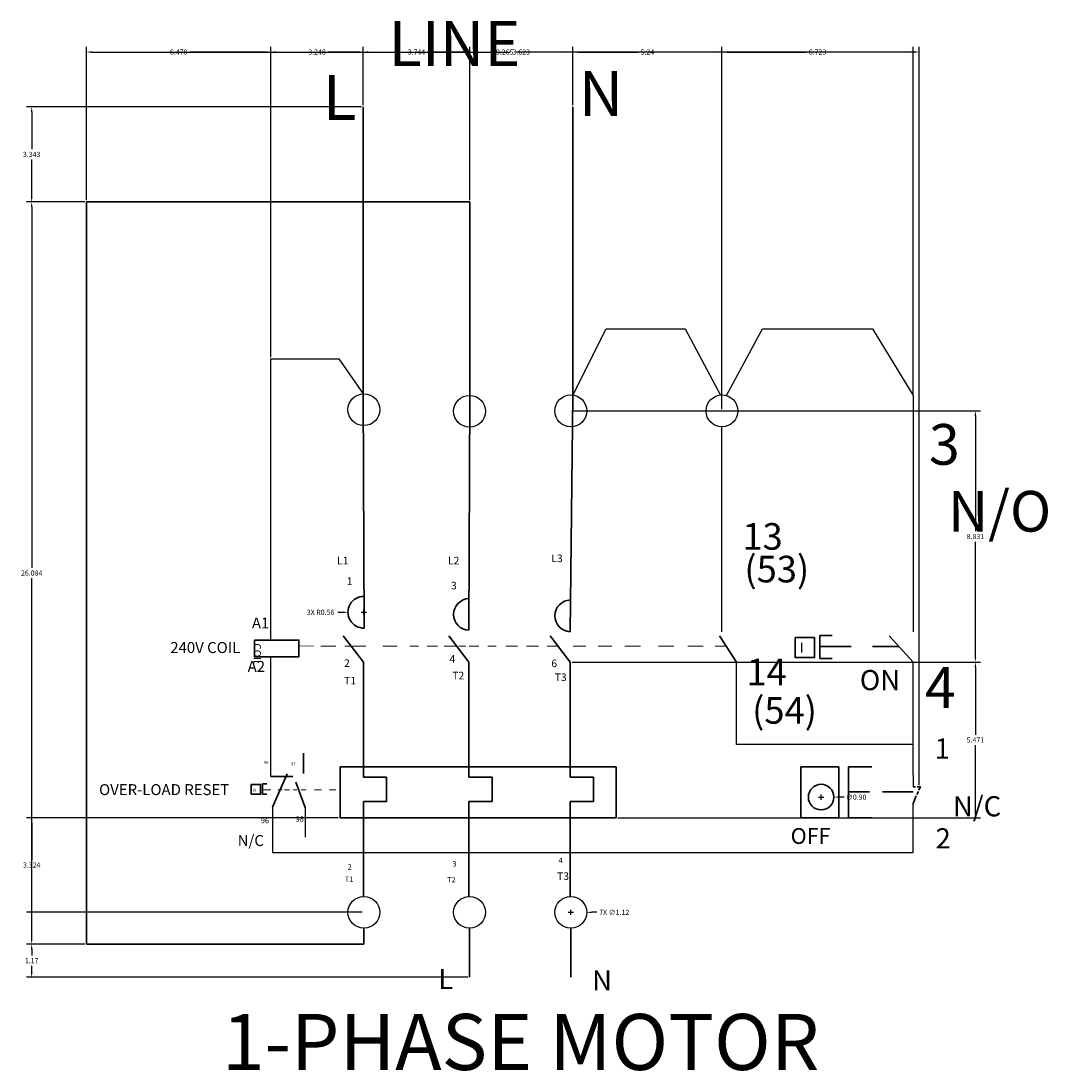
# Model space of a CAD drawing. Units: inches. Extents: x 14.6 to 50.7, y 1.8 to 38.7.
import ezdxf

# ---------------------------------------------------------------- set-up
doc = ezdxf.new("R2010")
doc.units = ezdxf.units.IN
doc.header["$MEASUREMENT"] = 0
for name, color, linetype, lineweight in [('A-ANNO-DIMS', 2, 'Continuous', 18), ('E-ANNO-TEXT', 7, 'Continuous', 18), ('E-CTRL-PBTN', 7, 'Continuous', 30), ('E-CTRL-WIRE', 4, 'Continuous', 25), ('E-EQPM-LINK', 8, 'Continuous', 18), ('E-POWR-CONT', 7, 'Continuous', 30), ('E-POWR-OVLD', 7, 'Continuous', 30), ('E-POWR-TERM', 2, 'Continuous', 25), ('E-POWR-WIRE', 1, 'Continuous', 35)]:
    doc.layers.add(name, color=color, linetype=linetype, lineweight=lineweight)
doc.styles.get("Standard").update_dxf_attribs({"font": 'arial.ttf'})
doc.dimstyles.get("Standard").update_dxf_attribs({"dimtxt": 0.18, "dimasz": 0.18, "dimexe": 0.18, "dimexo": 0.0625, "dimgap": 0.09, "dimtad": 0, "dimtih": 1, "dimtoh": 1, "dimdec": 4, "dimzin": 0, "dimdsep": 46, "dimtxsty": 'Standard', "dimcen": 0.09, "dimadec": 0, "dimazin": 0, "dimtfac": 1, "dimtdec": 4, "dimtofl": 0, "dimtmove": 0, "dimatfit": 3, "dimfxl": 1, "dimtolj": 1, "dimtzin": 0, "dimarcsym": 0})

# ---------------------------------------------------------------- blocks, each defined once
blk = doc.blocks.new('OL-HEATER-ELEMENT')
for p, q in [((0.817, 0.861), (0, 0.861)), ((0.817, 0), (0.817, 0.861)), ((0, 0), (0.817, 0))]:
    blk.add_line(p, q)
blk = doc.blocks.new('WIRING-TERMINAL')
blk.add_circle((0, 0), 0.558)
blk = doc.blocks.new('*D3')
at = {"layer": 'A-ANNO-DIMS', "color": 0, "lineweight": -2, "transparency": 16777216}
for p, q in [((16.913, 32.366), (16.913, 37.754)), ((46.178, 11.804), (46.178, 37.754)), ((17.093, 37.574), (31.08, 37.574)), ((45.998, 37.574), (32.011, 37.574))]:
    blk.add_line(p, q, dxfattribs=at)
at = {"layer": 'A-ANNO-DIMS', "color": 0, "transparency": 16777216}
for points in [[(17.093, 37.604), (17.093, 37.544), (16.913, 37.574)], [(45.998, 37.604), (45.998, 37.544), (46.178, 37.574)]]:
    blk.add_solid(points, dxfattribs=at)
at = {"layer": 'Defpoints', "color": 0, "transparency": 16777216}
for p in [(46.178, 37.574), (16.913, 32.303), (46.178, 11.741)]:
    blk.add_point(p, dxfattribs=at)
at = {"layer": 'A-ANNO-DIMS', "color": 0, "transparency": 16777216, "insert": (31.546, 37.574), "char_height": 0.18, "attachment_point": 5}
blk.add_mtext('\\A1;29.265', dxfattribs=at)
blk = doc.blocks.new('*D4')
at = {"layer": 'A-ANNO-DIMS', "color": 0, "lineweight": -2, "transparency": 16777216}
for p, q in [((16.851, 32.303), (14.806, 32.303)), ((14.986, 32.123), (14.986, 19.443)), ((14.986, 6.399), (14.986, 19.079)), ((16.851, 6.219), (14.806, 6.219))]:
    blk.add_line(p, q, dxfattribs=at)
at = {"layer": 'A-ANNO-DIMS', "color": 0, "transparency": 16777216}
for points in [[(14.956, 32.123), (15.016, 32.123), (14.986, 32.303)], [(14.956, 6.399), (15.016, 6.399), (14.986, 6.219)]]:
    blk.add_solid(points, dxfattribs=at)
at = {"layer": 'Defpoints', "color": 0, "transparency": 16777216}
for p in [(14.986, 32.303), (16.913, 32.303), (16.913, 6.219)]:
    blk.add_point(p, dxfattribs=at)
at = {"layer": 'A-ANNO-DIMS', "color": 0, "transparency": 16777216, "insert": (14.986, 19.261), "char_height": 0.18, "attachment_point": 5}
blk.add_mtext('\\A1;26.084', dxfattribs=at)
blk = doc.blocks.new('*D5')
at = {"layer": 'A-ANNO-DIMS', "color": 0, "lineweight": -2, "transparency": 16777216}
for p, q in [((26.576, 35.647), (14.806, 35.647)), ((14.986, 35.467), (14.986, 34.157)), ((14.986, 32.483), (14.986, 33.793)), ((16.851, 32.303), (14.806, 32.303))]:
    blk.add_line(p, q, dxfattribs=at)
at = {"layer": 'A-ANNO-DIMS', "color": 0, "transparency": 16777216}
for points in [[(14.956, 35.467), (15.016, 35.467), (14.986, 35.647)], [(14.956, 32.483), (15.016, 32.483), (14.986, 32.303)]]:
    blk.add_solid(points, dxfattribs=at)
at = {"layer": 'Defpoints', "color": 0, "transparency": 16777216}
for p in [(14.986, 35.647), (26.639, 35.647), (16.913, 32.303)]:
    blk.add_point(p, dxfattribs=at)
at = {"layer": 'A-ANNO-DIMS', "color": 0, "transparency": 16777216, "insert": (14.986, 33.975), "char_height": 0.18, "attachment_point": 5}
blk.add_mtext('\\A1;3.343', dxfattribs=at)
blk = doc.blocks.new('*D6')
at = {"layer": 'A-ANNO-DIMS', "color": 0, "lineweight": -2, "transparency": 16777216}
for p, q in [((16.851, 6.219), (14.806, 6.219)), ((14.986, 6.039), (14.986, 5.816)), ((14.986, 5.233), (14.986, 5.456)), ((30.313, 5.053), (14.806, 5.053))]:
    blk.add_line(p, q, dxfattribs=at)
at = {"layer": 'A-ANNO-DIMS', "color": 0, "transparency": 16777216}
for points in [[(14.956, 6.039), (15.016, 6.039), (14.986, 6.219)], [(14.956, 5.233), (15.016, 5.233), (14.986, 5.053)]]:
    blk.add_solid(points, dxfattribs=at)
at = {"layer": 'Defpoints', "color": 0, "transparency": 16777216}
for p in [(14.986, 6.219), (16.913, 6.219), (30.375, 5.053)]:
    blk.add_point(p, dxfattribs=at)
at = {"layer": 'A-ANNO-DIMS', "color": 0, "transparency": 16777216, "insert": (14.986, 5.636), "char_height": 0.18, "attachment_point": 5}
blk.add_mtext('\\A1;1.17', dxfattribs=at)
blk = doc.blocks.new('*D7')
at = {"layer": 'A-ANNO-DIMS', "color": 0, "lineweight": -2, "transparency": 16777216}
for p, q in [((16.913, 32.366), (16.913, 37.754)), ((23.391, 26.852), (23.391, 37.754)), ((17.093, 37.574), (19.758, 37.574)), ((23.211, 37.574), (20.546, 37.574))]:
    blk.add_line(p, q, dxfattribs=at)
at = {"layer": 'A-ANNO-DIMS', "color": 0, "transparency": 16777216}
for points in [[(17.093, 37.604), (17.093, 37.544), (16.913, 37.574)], [(23.211, 37.604), (23.211, 37.544), (23.391, 37.574)]]:
    blk.add_solid(points, dxfattribs=at)
at = {"layer": 'Defpoints', "color": 0, "transparency": 16777216}
for p in [(23.391, 37.574), (16.913, 32.303), (23.391, 26.79)]:
    blk.add_point(p, dxfattribs=at)
at = {"layer": 'A-ANNO-DIMS', "color": 0, "transparency": 16777216, "insert": (20.152, 37.574), "char_height": 0.18, "attachment_point": 5}
blk.add_mtext('\\A1;6.478', dxfattribs=at)
blk = doc.blocks.new('*D8')
at = {"layer": 'A-ANNO-DIMS', "color": 0, "lineweight": -2, "transparency": 16777216}
for p, q in [((23.391, 26.852), (23.391, 37.754)), ((26.639, 35.709), (26.639, 37.754)), ((23.571, 37.574), (24.621, 37.574)), ((26.459, 37.574), (25.409, 37.574))]:
    blk.add_line(p, q, dxfattribs=at)
at = {"layer": 'A-ANNO-DIMS', "color": 0, "transparency": 16777216}
for points in [[(23.571, 37.604), (23.571, 37.544), (23.391, 37.574)], [(26.459, 37.604), (26.459, 37.544), (26.639, 37.574)]]:
    blk.add_solid(points, dxfattribs=at)
at = {"layer": 'Defpoints', "color": 0, "transparency": 16777216}
for p in [(26.639, 37.574), (26.639, 35.647), (23.391, 26.79)]:
    blk.add_point(p, dxfattribs=at)
at = {"layer": 'A-ANNO-DIMS', "color": 0, "transparency": 16777216, "insert": (25.015, 37.574), "char_height": 0.18, "attachment_point": 5}
blk.add_mtext('\\A1;3.248', dxfattribs=at)
blk = doc.blocks.new('*D9')
at = {"layer": 'A-ANNO-DIMS', "color": 0, "lineweight": -2, "transparency": 16777216}
for p, q in [((26.639, 35.709), (26.639, 37.754)), ((30.383, 32.366), (30.383, 37.754)), ((26.819, 37.574), (28.117, 37.574)), ((30.203, 37.574), (28.904, 37.574))]:
    blk.add_line(p, q, dxfattribs=at)
at = {"layer": 'A-ANNO-DIMS', "color": 0, "transparency": 16777216}
for points in [[(26.819, 37.604), (26.819, 37.544), (26.639, 37.574)], [(30.203, 37.604), (30.203, 37.544), (30.383, 37.574)]]:
    blk.add_solid(points, dxfattribs=at)
at = {"layer": 'Defpoints', "color": 0, "transparency": 16777216}
for p in [(30.383, 37.574), (26.639, 35.647), (30.383, 32.303)]:
    blk.add_point(p, dxfattribs=at)
at = {"layer": 'A-ANNO-DIMS', "color": 0, "transparency": 16777216, "insert": (28.511, 37.574), "char_height": 0.18, "attachment_point": 5}
blk.add_mtext('\\A1;3.744', dxfattribs=at)
blk = doc.blocks.new('*D10')
at = {"layer": 'A-ANNO-DIMS', "color": 0, "lineweight": -2, "transparency": 16777216}
for p, q in [((30.383, 32.366), (30.383, 37.754)), ((34.006, 35.709), (34.006, 37.754)), ((30.563, 37.574), (31.801, 37.574)), ((33.826, 37.574), (32.588, 37.574))]:
    blk.add_line(p, q, dxfattribs=at)
at = {"layer": 'A-ANNO-DIMS', "color": 0, "transparency": 16777216}
for points in [[(30.563, 37.604), (30.563, 37.544), (30.383, 37.574)], [(33.826, 37.604), (33.826, 37.544), (34.006, 37.574)]]:
    blk.add_solid(points, dxfattribs=at)
at = {"layer": 'Defpoints', "color": 0, "transparency": 16777216}
for p in [(34.006, 37.574), (34.006, 35.647), (30.383, 32.303)]:
    blk.add_point(p, dxfattribs=at)
at = {"layer": 'A-ANNO-DIMS', "color": 0, "transparency": 16777216, "insert": (32.194, 37.574), "char_height": 0.18, "attachment_point": 5}
blk.add_mtext('\\A1;3.623', dxfattribs=at)
blk = doc.blocks.new('*D11')
at = {"layer": 'A-ANNO-DIMS', "color": 0, "lineweight": -2, "transparency": 16777216}
for p, q in [((34.006, 35.709), (34.006, 37.754)), ((39.246, 25.023), (39.246, 37.754)), ((34.186, 37.574), (36.303, 37.574)), ((39.066, 37.574), (36.949, 37.574))]:
    blk.add_line(p, q, dxfattribs=at)
at = {"layer": 'A-ANNO-DIMS', "color": 0, "transparency": 16777216}
for points in [[(34.186, 37.604), (34.186, 37.544), (34.006, 37.574)], [(39.066, 37.604), (39.066, 37.544), (39.246, 37.574)]]:
    blk.add_solid(points, dxfattribs=at)
at = {"layer": 'Defpoints', "color": 0, "transparency": 16777216}
for p in [(39.246, 37.574), (34.006, 35.647), (39.246, 24.961)]:
    blk.add_point(p, dxfattribs=at)
at = {"layer": 'A-ANNO-DIMS', "color": 0, "transparency": 16777216, "insert": (36.626, 37.574), "char_height": 0.18, "attachment_point": 5}
blk.add_mtext('\\A1;5.24', dxfattribs=at)
blk = doc.blocks.new('*D12')
at = {"layer": 'A-ANNO-DIMS', "color": 0, "lineweight": -2, "transparency": 16777216}
for p, q in [((39.246, 25.023), (39.246, 37.754)), ((45.969, 25.558), (45.969, 37.754)), ((39.426, 37.574), (42.213, 37.574)), ((45.789, 37.574), (43.002, 37.574))]:
    blk.add_line(p, q, dxfattribs=at)
at = {"layer": 'A-ANNO-DIMS', "color": 0, "transparency": 16777216}
for points in [[(39.426, 37.604), (39.426, 37.544), (39.246, 37.574)], [(45.789, 37.604), (45.789, 37.544), (45.969, 37.574)]]:
    blk.add_solid(points, dxfattribs=at)
at = {"layer": 'Defpoints', "color": 0, "transparency": 16777216}
for p in [(45.969, 37.574), (45.969, 25.496), (39.246, 24.961)]:
    blk.add_point(p, dxfattribs=at)
at = {"layer": 'A-ANNO-DIMS', "color": 0, "transparency": 16777216, "insert": (42.608, 37.574), "char_height": 0.18, "attachment_point": 5}
blk.add_mtext('\\A1;6.723', dxfattribs=at)
blk = doc.blocks.new('*D13')
at = {"layer": 'A-ANNO-DIMS', "color": 0, "lineweight": -2, "transparency": 16777216}
for p, q in [((25.762, 10.658), (14.806, 10.658)), ((14.986, 10.478), (14.986, 9.178)), ((14.986, 7.514), (14.986, 8.814)), ((26.599, 7.334), (14.806, 7.334))]:
    blk.add_line(p, q, dxfattribs=at)
at = {"layer": 'A-ANNO-DIMS', "color": 0, "transparency": 16777216}
for points in [[(14.956, 10.478), (15.016, 10.478), (14.986, 10.658)], [(14.956, 7.514), (15.016, 7.514), (14.986, 7.334)]]:
    blk.add_solid(points, dxfattribs=at)
at = {"layer": 'Defpoints', "color": 0, "transparency": 16777216}
for p in [(14.986, 10.658), (25.824, 10.658), (26.662, 7.334)]:
    blk.add_point(p, dxfattribs=at)
at = {"layer": 'A-ANNO-DIMS', "color": 0, "transparency": 16777216, "insert": (14.986, 8.996), "char_height": 0.18, "attachment_point": 5}
blk.add_mtext('\\A1;3.324', dxfattribs=at)
blk = doc.blocks.new('*D14')
at = {"layer": 'A-ANNO-DIMS', "color": 0, "lineweight": -2, "transparency": 16777216}
for p, q in [((33.981, 16.129), (48.336, 16.129)), ((48.156, 15.949), (48.156, 13.576)), ((48.156, 10.838), (48.156, 13.212)), ((35.589, 10.658), (48.336, 10.658))]:
    blk.add_line(p, q, dxfattribs=at)
at = {"layer": 'A-ANNO-DIMS', "color": 0, "transparency": 16777216}
for points in [[(48.126, 15.949), (48.186, 15.949), (48.156, 16.129)], [(48.126, 10.838), (48.186, 10.838), (48.156, 10.658)]]:
    blk.add_solid(points, dxfattribs=at)
at = {"layer": 'Defpoints', "color": 0, "transparency": 16777216}
for p in [(33.918, 16.129), (48.156, 16.129), (35.526, 10.658)]:
    blk.add_point(p, dxfattribs=at)
at = {"layer": 'A-ANNO-DIMS', "color": 0, "transparency": 16777216, "insert": (48.156, 13.394), "char_height": 0.18, "attachment_point": 5}
blk.add_mtext('\\A1;5.471', dxfattribs=at)
blk = doc.blocks.new('*D15')
at = {"layer": 'A-ANNO-DIMS', "color": 0, "lineweight": -2, "transparency": 16777216}
for p, q in [((33.999, 24.961), (48.336, 24.961)), ((48.156, 24.781), (48.156, 20.727)), ((48.156, 16.309), (48.156, 20.363)), ((33.981, 16.129), (48.336, 16.129))]:
    blk.add_line(p, q, dxfattribs=at)
at = {"layer": 'A-ANNO-DIMS', "color": 0, "transparency": 16777216}
for points in [[(48.126, 24.781), (48.186, 24.781), (48.156, 24.961)], [(48.126, 16.309), (48.186, 16.309), (48.156, 16.129)]]:
    blk.add_solid(points, dxfattribs=at)
at = {"layer": 'Defpoints', "color": 0, "transparency": 16777216}
for p in [(33.936, 24.961), (48.156, 24.961), (33.918, 16.129)]:
    blk.add_point(p, dxfattribs=at)
at = {"layer": 'A-ANNO-DIMS', "color": 0, "transparency": 16777216, "insert": (48.156, 20.545), "char_height": 0.18, "attachment_point": 5}
blk.add_mtext('\\A1;8.831', dxfattribs=at)
blk = doc.blocks.new('*D16')
at = {"layer": 'A-ANNO-DIMS', "color": 0, "lineweight": -2, "transparency": 16777216}
for p, q in [((25.744, 17.88), (25.924, 17.88)), ((26.572, 17.883), (26.752, 17.883)), ((26.662, 17.793), (26.662, 17.973))]:
    blk.add_line(p, q, dxfattribs=at)
at = {"layer": 'A-ANNO-DIMS', "color": 0, "transparency": 16777216}
blk.add_solid([(25.923, 17.91), (25.924, 17.85), (26.104, 17.881)], dxfattribs=at)
at = {"layer": 'Defpoints', "color": 0, "transparency": 16777216}
for p in [(26.104, 17.881), (26.662, 17.883)]:
    blk.add_point(p, dxfattribs=at)
at = {"layer": 'A-ANNO-DIMS', "color": 0, "transparency": 16777216, "insert": (25.14, 17.88), "char_height": 0.18, "attachment_point": 5}
blk.add_mtext('\\A1;3X R0.56', dxfattribs=at)
blk = doc.blocks.new('*D17')
at = {"layer": 'A-ANNO-DIMS', "color": 0, "lineweight": -2, "transparency": 16777216}
for p, q in [((33.936, 7.244), (33.936, 7.424)), ((33.846, 7.334), (34.026, 7.334)), ((34.854, 7.334), (34.674, 7.334))]:
    blk.add_line(p, q, dxfattribs=at)
at = {"layer": 'A-ANNO-DIMS', "color": 0, "transparency": 16777216}
blk.add_solid([(34.674, 7.364), (34.674, 7.304), (34.494, 7.334)], dxfattribs=at)
at = {"layer": 'Defpoints', "color": 0, "transparency": 16777216}
for p in [(33.378, 7.335), (34.494, 7.334)]:
    blk.add_point(p, dxfattribs=at)
at = {"layer": 'A-ANNO-DIMS', "color": 0, "transparency": 16777216, "insert": (35.463, 7.334), "char_height": 0.18, "attachment_point": 5}
blk.add_mtext('\\A1;7X ∅1.12', dxfattribs=at)
blk = doc.blocks.new('*D18')
at = {"layer": 'A-ANNO-DIMS', "color": 0, "lineweight": -2, "transparency": 16777216}
for p, q in [((42.733, 11.294), (42.733, 11.474)), ((42.643, 11.384), (42.823, 11.384)), ((43.543, 11.384), (43.363, 11.384))]:
    blk.add_line(p, q, dxfattribs=at)
at = {"layer": 'A-ANNO-DIMS', "color": 0, "transparency": 16777216}
blk.add_solid([(43.363, 11.414), (43.363, 11.354), (43.183, 11.384)], dxfattribs=at)
at = {"layer": 'Defpoints', "color": 0, "transparency": 16777216}
for p in [(42.284, 11.384), (43.183, 11.384)]:
    blk.add_point(p, dxfattribs=at)
at = {"layer": 'A-ANNO-DIMS', "color": 0, "transparency": 16777216, "insert": (43.964, 11.384), "char_height": 0.18, "attachment_point": 5}
blk.add_mtext('\\A1;∅0.90', dxfattribs=at)

msp = doc.modelspace()

# ---------------------------------------------------------------- linework, layer by layer
at = {"layer": 'E-CTRL-PBTN'}
for p, q in [((42.692, 17.0629), (42.692, 16.2592)), ((42.692, 17.0629), (43.1203, 17.0629)), ((45.9692, 16.1292), (45.1231, 17.0516)), ((43.7887, 16.676), (42.692, 16.676)), ((45.4676, 16.676), (44.5408, 16.676)), ((42.692, 16.2592), (43.1203, 16.2592)), ((44.5217, 12.4427), (43.6936, 12.4427)), ((43.6936, 12.4427), (43.6936, 10.6582)), ((43.6936, 11.5739), (44.4364, 11.5739)), ((44.891, 11.5739), (45.9692, 11.5724)), ((45.9692, 11.7412), (46.0491, 11.7412)), ((46.1013, 11.4785), (46.1509, 11.586)), ((46.1086, 11.7412), (46.1778, 11.7412)), ((46.1705, 11.6311), (46.2289, 11.7595)), ((46.1991, 11.7412), (46.2286, 11.7412)), ((45.9692, 11.1583), (46.0787, 11.4258)), ((43.6936, 10.6582), (44.5217, 10.6582))]:
    msp.add_line(p, q, dxfattribs=at)
for points in [[(41.8221, 16.9917), (42.4989, 16.9917), (42.4989, 16.2856), (41.8221, 16.2856)], [(42.016, 12.4427), (43.355, 12.4427), (43.355, 10.6582), (42.016, 10.6582)]]:
    msp.add_lwpolyline(points, close=True, dxfattribs=at)
msp.add_circle((42.7334, 11.3839), 0.4493, dxfattribs=at)
at = {"layer": 'E-CTRL-WIRE'}
for p, q in [((34.006, 25.5143), (35.1735, 27.8392)), ((35.1735, 27.8392), (37.9599, 27.8392)), ((37.9599, 27.8392), (39.1914, 25.516)), ((39.4041, 25.4958), (40.6684, 27.8392)), ((40.6684, 27.8392), (44.5431, 27.8392)), ((44.5431, 27.8392), (45.9692, 25.4958)), ((23.3909, 16.9065), (23.3909, 26.7895)), ((23.3909, 26.7895), (25.7823, 26.7895)), ((25.7823, 26.7895), (26.6386, 25.558)), ((45.9692, 25.4958), (45.9692, 21.862)), ((39.2338, 24.4025), (39.2338, 17.1985)), ((45.9692, 21.862), (45.9692, 17.1985)), ((23.3909, 12.1107), (23.3909, 16.3173)), ((39.7587, 13.2359), (39.7587, 16.1292)), ((45.9692, 12.155), (45.9692, 16.1292)), ((45.9692, 13.2359), (39.7587, 13.2359)), ((45.9692, 12.155), (45.9692, 11.7412)), ((45.9692, 9.4343), (45.9692, 11.1583)), ((23.4508, 11.0282), (23.4508, 9.4343)), ((24.5996, 11.0239), (24.5996, 9.9713)), ((23.4508, 9.4343), (40.7008, 9.4343)), ((40.7008, 9.4343), (45.9692, 9.4343))]:
    msp.add_line(p, q, dxfattribs=at)
at = {"layer": 'E-EQPM-LINK'}
for p, q in [((24.8889, 16.6877), (24.3785, 16.6986)), ((25.6805, 16.6877), (25.1464, 16.6877)), ((26.7342, 16.6877), (25.9957, 16.6877)), ((27.8354, 16.6877), (27.3303, 16.6877)), ((28.5862, 16.6877), (28.2799, 16.6877)), ((29.2552, 16.6877), (28.8877, 16.6877)), ((29.9334, 16.6877), (29.4814, 16.6877)), ((30.2431, 16.6877), (30.0052, 16.6877)), ((30.7043, 16.6877), (30.3624, 16.6877)), ((31.3086, 16.6877), (31.0196, 16.6877)), ((32.0572, 16.6877), (31.657, 16.6877)), ((32.8058, 16.6877), (32.3759, 16.6877)), ((33.4896, 16.6877), (33.1097, 16.6877)), ((34.0175, 16.6877), (34.4685, 16.6877)), ((34.8999, 16.6877), (35.3803, 16.6877)), ((35.8313, 16.6877), (36.3804, 16.6877)), ((37.0213, 16.6877), (37.5615, 16.6877)), ((38.0527, 16.6877), (38.5929, 16.6877)), ((39.0143, 16.6877), (39.3961, 16.6861)), ((23.3974, 11.6358), (23.0955, 11.6358)), ((23.7856, 11.6358), (23.6396, 11.6358)), ((24.0511, 11.6358), (23.8747, 11.6358)), ((24.304, 11.6358), (24.1757, 11.6358)), ((24.6353, 11.6358), (24.4554, 11.6358)), ((25.171, 11.6358), (24.931, 11.6358)), ((25.673, 11.6358), (25.4547, 11.6358))]:
    msp.add_line(p, q, dxfattribs=at)
at = {"layer": 'E-POWR-CONT'}
for p, q in [((26.6435, 16.1292), (25.9361, 17.0516)), ((30.3571, 16.1292), (29.6497, 17.0516)), ((33.918, 16.1292), (33.2106, 17.0516)), ((39.7587, 16.1292), (39.1581, 17.0516))]:
    msp.add_line(p, q, dxfattribs=at)
msp.add_lwpolyline([(22.8176, 16.9065), (24.3785, 16.9065), (24.3785, 16.3173), (22.8176, 16.3173)], close=True, dxfattribs=at)
for centre, start, end in [((26.6617, 17.8832), 88.90529, 271.63696), ((30.3753, 17.8053), 91.8333, 267.75999), ((33.9361, 17.756), 91.40433, 267.26604)]:
    msp.add_arc(centre, 0.5582, start, end, dxfattribs=at)
at = {"layer": 'E-POWR-OVLD'}
for p, q in [((24.5382, 12.9269), (24.5382, 12.2172)), ((23.4508, 11.0282), (23.9713, 12.2057)), ((23.0955, 11.8489), (23.0955, 11.4824)), ((23.0955, 11.8489), (23.2468, 11.8489)), ((24.162, 12.1107), (23.3909, 12.1107)), ((24.5996, 11.0239), (24.2669, 11.9102)), ((23.0955, 11.4824), (23.2468, 11.4824))]:
    msp.add_line(p, q, dxfattribs=at)
for points in [[(25.8242, 12.4427), (35.5264, 12.4427), (35.5264, 10.6582), (25.8242, 10.6582)], [(22.7036, 11.8278), (23.0323, 11.8278), (23.0323, 11.4872), (22.7036, 11.4872)]]:
    msp.add_lwpolyline(points, close=True, dxfattribs=at)
at = {"layer": 'E-POWR-WIRE'}
for p, q in [((26.6386, 25.558), (26.6386, 35.6466)), ((34.006, 25.5143), (34.006, 35.6466)), ((30.3828, 32.3033), (16.9133, 32.3033)), ((16.9133, 32.3033), (16.9133, 6.2188)), ((30.3828, 25.5042), (30.3828, 32.3033)), ((26.6386, 25.558), (26.6776, 17.3253)), ((30.3828, 25.5042), (30.3534, 17.2476)), ((34.006, 25.5143), (33.9095, 17.1985)), ((26.6435, 12.0861), (26.6435, 16.1292)), ((30.3571, 12.0861), (30.3571, 16.1292)), ((33.918, 12.0861), (33.918, 16.1292)), ((26.6435, 7.8922), (26.6435, 11.2247)), ((30.3571, 7.8922), (30.3571, 11.2247)), ((33.918, 7.8922), (33.918, 11.2247)), ((26.6617, 6.2188), (26.6617, 6.7762)), ((30.3753, 6.2188), (30.3753, 6.7762)), ((33.9361, 6.2188), (33.9361, 6.7762)), ((16.9133, 6.2188), (20.0275, 6.2188)), ((20.0275, 6.2188), (26.6617, 6.2188)), ((30.3753, 6.2188), (30.3753, 5.053)), ((33.9361, 6.2188), (33.9361, 5.053))]:
    msp.add_line(p, q, dxfattribs=at)

# ---------------------------------------------------------------- block references
at = {"layer": 'E-POWR-OVLD'}
for p in [(26.6435, 11.2247), (30.3571, 11.2247), (33.918, 11.2247)]:
    msp.add_blockref('OL-HEATER-ELEMENT', p, dxfattribs=at)
at = {"layer": 'E-POWR-TERM'}
for p in [(26.6617, 25.0003), (30.3753, 24.9461), (33.9361, 24.9605), (39.246, 24.9605), (26.6617, 7.3343), (30.3753, 7.3343), (33.9361, 7.3343)]:
    msp.add_blockref('WIRING-TERMINAL', p, dxfattribs=at)

# ---------------------------------------------------------------- texts
at = {"layer": 'E-ANNO-TEXT'}
for s, height, p in [('LINE', 1.58446, (27.5253, 37.0804)), ('L', 1.5845, (25.2238, 35.1868)), ('N', 1.5845, (34.2144, 35.321)), ('3', 1.431, (46.5229, 23.0662)), ('N/O', 1.43097, (47.1958, 20.7153)), ('13', 0.935, (39.9665, 20.0806)), ('(53)', 0.935, (40.037, 18.9318)), ('L1', 0.26703, (25.7174, 19.5644)), ('L2', 0.26703, (29.619, 19.5644)), ('L3', 0.26703, (33.2502, 19.6435)), ('1', 0.267, (26.0578, 18.8395)), ('3', 0.267, (29.7243, 18.6861)), ('A1', 0.38546, (22.7277, 17.3108)), ('240V COIL', 0.38546, (19.8568, 16.4485)), ('I', 0.3488, (41.9781, 16.4624)), ('4', 0.267, (29.6723, 16.1071)), ('14', 0.935, (40.1103, 15.3137)), ('A2', 0.38546, (22.5784, 15.7852)), ('2', 0.267, (25.9663, 15.9586)), ('6', 0.267, (33.2508, 15.9525)), ('4', 1.431, (46.3827, 14.5214)), ('T1', 0.26703, (25.9663, 15.3431)), ('T2', 0.26703, (29.7679, 15.5235)), ('T3', 0.26703, (33.3678, 15.4635)), ('ON', 0.70872, (44.0945, 15.1429)), ('(54)', 0.935, (40.3082, 13.9656)), ('1', 0.7087, (46.7225, 12.7374)), ('OVER-LOAD RESET', 0.385456, (17.3559, 11.4538)), ('N/C', 0.70872, (47.3672, 10.7079)), ('98', 0.19054, (24.2633, 10.5187)), ('96', 0.19054, (23.0413, 10.466)), ('N/C', 0.38546, (22.226, 9.6645)), ('OFF', 0.55594, (41.6638, 9.7388)), ('2', 0.7087, (46.7547, 9.5804)), ('4', 0.1905, (33.5041, 9.0622)), ('2', 0.1905, (26.0893, 8.8382)), ('3', 0.1905, (29.7741, 8.9441)), ('T1', 0.19054, (25.9949, 8.3999)), ('T2', 0.19054, (29.5884, 8.3875)), ('T3', 0.26703, (33.4535, 8.4719)), ('L', 0.7087, (29.2777, 4.6384)), ('N', 0.7087, (34.6827, 4.5867)), ('1-PHASE MOTOR', 1.970344, (21.6784, 1.7915))]:
    msp.add_text(s, height=height, dxfattribs=at).set_placement(p)
for s, height, rotation, p in [('COIL', 0.25726, 270, (22.7858, 16.7881)), ('96', 0.1067, 2.24418, (23.1489, 12.547)), ('97', 0.1067, 2.24418, (24.0993, 12.4958)), ('R', 0.1067, 2.24418, (22.7743, 11.5677))]:
    msp.add_text(s, height=height, rotation=rotation, dxfattribs=at).set_placement(p)

# ---------------------------------------------------------------- dimensions: what is measured, and where the dimension line sits
at = {"layer": 'A-ANNO-DIMS'}
for base, p1, p2, override, picture, middle in [((46.17785, 37.57409), (16.91328, 32.30334), (46.17785, 11.74115), {"dimdec": 3, "dimlfac": 1, "dimrnd": 0, "dimzin": 0, "dimdsep": 46, "dimlunit": 2}, '*D3', (31.54556, 37.57409)), ((23.3909, 37.5741), (16.9133, 32.3033), (23.3909, 26.7895), {"dimdec": 3, "dimlfac": 1, "dimrnd": 0, "dimzin": 0, "dimdsep": 46, "dimlunit": 2}, '*D7', (20.1521, 37.5741)), ((26.6386, 37.5741), (23.3909, 26.7895), (26.6386, 35.6466), {"dimdec": 3, "dimlfac": 1, "dimrnd": 0, "dimzin": 0, "dimdsep": 46, "dimlunit": 2}, '*D8', (25.0148, 37.5741)), ((30.3828, 37.5741), (26.6386, 35.6466), (30.3828, 32.3033), {"dimdec": 3, "dimlfac": 1, "dimrnd": 0, "dimzin": 0, "dimdsep": 46, "dimlunit": 2}, '*D9', (28.5107, 37.5741)), ((34.006, 37.5741), (30.3828, 32.3033), (34.006, 35.6466), {"dimdec": 3, "dimlfac": 1, "dimrnd": 0, "dimzin": 0, "dimdsep": 46, "dimlunit": 2}, '*D10', (32.1944, 37.5741)), ((39.246, 37.5741), (34.006, 35.6466), (39.246, 24.9605), {"dimdec": 2, "dimlfac": 1, "dimrnd": 0, "dimzin": 0, "dimdsep": 46, "dimlunit": 2}, '*D11', (36.626, 37.5741)), ((45.9692, 37.5741), (39.246, 24.9605), (45.9692, 25.4958), {"dimdec": 3, "dimlfac": 1, "dimrnd": 0, "dimzin": 0, "dimdsep": 46, "dimlunit": 2}, '*D12', (42.6076, 37.5741))]:
    dim = msp.add_linear_dim(base=base, p1=p1, p2=p2, dimstyle='Standard', override=override, dxfattribs=at)
    dim.commit()
    dim.dimension.update_dxf_attribs({"geometry": picture, "text_midpoint": middle})
for base, p1, p2, override, picture, middle in [((14.9858, 35.6466), (16.9133, 32.3033), (26.6386, 35.6466), {"dimdec": 3, "dimlfac": 1, "dimrnd": 0, "dimzin": 0, "dimdsep": 46, "dimlunit": 2}, '*D5', (14.9858, 33.975)), ((14.985777, 32.30334), (16.913277, 6.218845), (16.913277, 32.30334), {"dimdec": 3, "dimlfac": 1, "dimrnd": 0, "dimzin": 0, "dimdsep": 46, "dimlunit": 2}, '*D4', (14.985777, 19.261092)), ((48.1564, 24.9605), (33.918, 16.1292), (33.9361, 24.9605), {"dimdec": 3, "dimlfac": 1, "dimrnd": 0, "dimzin": 0, "dimdsep": 46, "dimlunit": 2}, '*D15', (48.1564, 20.5448)), ((48.1564, 16.1292), (35.5264, 10.6582), (33.918, 16.1292), {"dimdec": 3, "dimlfac": 1, "dimrnd": 0, "dimzin": 0, "dimdsep": 46, "dimlunit": 2}, '*D14', (48.1564, 13.3937)), ((14.9858, 10.6582), (26.6617, 7.3343), (25.8242, 10.6582), {"dimdec": 3, "dimlfac": 1, "dimrnd": 0, "dimzin": 0, "dimdsep": 46, "dimlunit": 2}, '*D13', (14.9858, 8.9963)), ((14.9858, 6.2188), (30.3753, 5.053), (16.9133, 6.2188), {"dimdec": 2, "dimlfac": 1, "dimrnd": 0, "dimzin": 0, "dimdsep": 46, "dimlunit": 2}, '*D6', (14.9858, 5.6359))]:
    dim = msp.add_linear_dim(base=base, p1=p1, p2=p2, angle=90, dimstyle='Standard', override=override, dxfattribs=at)
    dim.commit()
    dim.dimension.update_dxf_attribs({"geometry": picture, "text_midpoint": middle})
dim = msp.add_radius_dim(center=(26.6617, 17.8832), mpoint=(26.1035, 17.881), text='3X <>', dimstyle='Standard', override={"dimdec": 2, "dimlfac": 1, "dimrnd": 0, "dimzin": 0, "dimdsep": 46, "dimlunit": 2}, dxfattribs=at)
dim.commit()
dim.dimension.update_dxf_attribs({"geometry": '*D16', "text_midpoint": (25.1403, 17.8796)})
dim = msp.add_diameter_dim_2p(p1=(42.2841, 11.3839), p2=(43.1828, 11.384), dimstyle='Standard', override={"dimdec": 2, "dimlfac": 1, "dimrnd": 0, "dimzin": 0, "dimdsep": 46, "dimlunit": 2}, dxfattribs=at)
dim.commit()
dim.dimension.update_dxf_attribs({"geometry": '*D18', "text_midpoint": (43.5428, 11.3841), "dimtype": 163})
dim = msp.add_diameter_dim_2p(p1=(33.378, 7.3347), p2=(34.4943, 7.334), text='7X <>', dimstyle='Standard', override={"dimdec": 2, "dimlfac": 1, "dimrnd": 0, "dimzin": 0, "dimdsep": 46, "dimlunit": 2}, dxfattribs=at)
dim.commit()
dim.dimension.update_dxf_attribs({"geometry": '*D17', "text_midpoint": (34.8543, 7.3338), "dimtype": 163})

doc.saveas('drawing.dxf')
